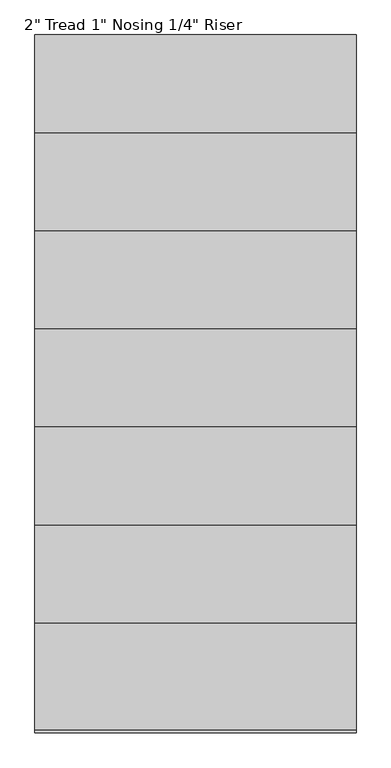
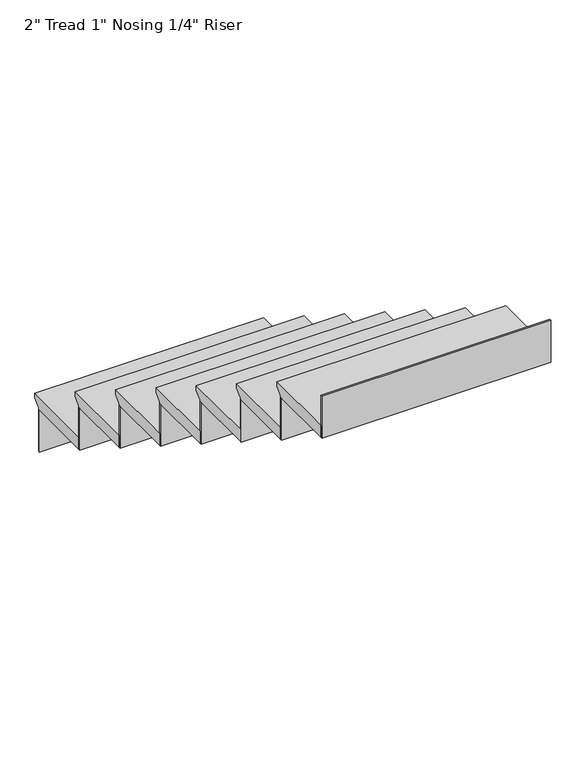
"""IFC4 building model written with IfcOpenShell, lengths in millimetres: stair flight geometry."""

from ifc_helpers import new_model, si_unit, frame, origin, place, context, project, spatial, polyline, outline, extrude, source, transform, mapped, element, save


def stair_flight_4fb3dba1(model_context):
    return source(origin(), model_context, "Body", "SweptSolid", [
        extrude(outline(polyline([(494.0027016, 8966.2), (798.8027016, 8966.2), (798.8027016, 8947.15), (773.4027016, 8921.75), (773.4027016, 8915.4), (494.0027016, 8915.4), (494.0027016, 8966.2)])), frame((8683.6260838, 0.0, 0.0), z_axis=(1.0, 0.0, 0.0), x_axis=(0.0, 1.0, 0.0)), (0.0, 0.0, 1.0), 914.4),
        extrude(outline(polyline([(8683.6260838, 767.0527016), (8683.6260838, 773.4027016), (9598.0260838, 773.4027016), (9598.0260838, 767.0527016), (8683.6260838, 767.0527016)])), frame((0.0, 0.0, 8737.6), z_axis=(0.0, 0.0, 1.0), x_axis=(1.0, 0.0, 0.0)), (0.0, 0.0, 1.0), 177.8),
        extrude(outline(polyline([(8683.6260838, 487.6527016), (8683.6260838, 494.0027016), (9598.0260838, 494.0027016), (9598.0260838, 487.6527016), (8683.6260838, 487.6527016)])), frame((0.0, 0.0, 8915.4), z_axis=(0.0, 0.0, 1.0), x_axis=(1.0, 0.0, 0.0)), (0.0, 0.0, 1.0), 177.8),
        extrude(outline(polyline([(214.6027016, 9144.0), (519.4027016, 9144.0), (519.4027016, 9124.95), (494.0027016, 9099.55), (494.0027016, 9093.2), (214.6027016, 9093.2), (214.6027016, 9144.0)])), frame((8683.6260838, 0.0, 0.0), z_axis=(1.0, 0.0, 0.0), x_axis=(0.0, 1.0, 0.0)), (0.0, 0.0, 1.0), 914.4),
        extrude(outline(polyline([(8683.6260838, 208.2527016), (8683.6260838, 214.6027016), (9598.0260838, 214.6027016), (9598.0260838, 208.2527016), (8683.6260838, 208.2527016)])), frame((0.0, 0.0, 9093.2), z_axis=(0.0, 0.0, 1.0), x_axis=(1.0, 0.0, 0.0)), (0.0, 0.0, 1.0), 177.8),
        extrude(outline(polyline([(-64.7972984, 9321.8), (240.0027016, 9321.8), (240.0027016, 9302.75), (214.6027016, 9277.35), (214.6027016, 9271.0), (-64.7972984, 9271.0), (-64.7972984, 9321.8)])), frame((8683.6260838, 0.0, 0.0), z_axis=(1.0, 0.0, 0.0), x_axis=(0.0, 1.0, 0.0)), (0.0, 0.0, 1.0), 914.4),
        extrude(outline(polyline([(8683.6260838, -71.1472984), (8683.6260838, -64.7972984), (9598.0260838, -64.7972984), (9598.0260838, -71.1472984), (8683.6260838, -71.1472984)])), frame((0.0, 0.0, 9271.0), z_axis=(0.0, 0.0, 1.0), x_axis=(1.0, 0.0, 0.0)), (0.0, 0.0, 1.0), 177.8),
        extrude(outline(polyline([(-344.1972984, 9499.6), (-39.3972984, 9499.6), (-39.3972984, 9480.55), (-64.7972984, 9455.15), (-64.7972984, 9448.8), (-344.1972984, 9448.8), (-344.1972984, 9499.6)])), frame((8683.6260838, 0.0, 0.0), z_axis=(1.0, 0.0, 0.0), x_axis=(0.0, 1.0, 0.0)), (0.0, 0.0, 1.0), 914.4),
        extrude(outline(polyline([(8683.6260838, -350.5472984), (8683.6260838, -344.1972984), (9598.0260838, -344.1972984), (9598.0260838, -350.5472984), (8683.6260838, -350.5472984)])), frame((0.0, 0.0, 9448.8), z_axis=(0.0, 0.0, 1.0), x_axis=(1.0, 0.0, 0.0)), (0.0, 0.0, 1.0), 177.8),
        extrude(outline(polyline([(-623.5972984, 9677.4), (-318.7972984, 9677.4), (-318.7972984, 9658.35), (-344.1972984, 9632.95), (-344.1972984, 9626.6), (-623.5972984, 9626.6), (-623.5972984, 9677.4)])), frame((8683.6260838, 0.0, 0.0), z_axis=(1.0, 0.0, 0.0), x_axis=(0.0, 1.0, 0.0)), (0.0, 0.0, 1.0), 914.4),
        extrude(outline(polyline([(8683.6260838, -629.9472984), (8683.6260838, -623.5972984), (9598.0260838, -623.5972984), (9598.0260838, -629.9472984), (8683.6260838, -629.9472984)])), frame((0.0, 0.0, 9626.6), z_axis=(0.0, 0.0, 1.0), x_axis=(1.0, 0.0, 0.0)), (0.0, 0.0, 1.0), 177.8),
        extrude(outline(polyline([(-902.9972984, 9855.2), (-598.1972984, 9855.2), (-598.1972984, 9836.15), (-623.5972984, 9810.75), (-623.5972984, 9804.4), (-902.9972984, 9804.4), (-902.9972984, 9855.2)])), frame((8683.6260838, 0.0, 0.0), z_axis=(1.0, 0.0, 0.0), x_axis=(0.0, 1.0, 0.0)), (0.0, 0.0, 1.0), 914.4),
        extrude(outline(polyline([(8683.6260838, -909.3472984), (8683.6260838, -902.9972984), (9598.0260838, -902.9972984), (9598.0260838, -909.3472984), (8683.6260838, -909.3472984)])), frame((0.0, 0.0, 9804.4), z_axis=(0.0, 0.0, 1.0), x_axis=(1.0, 0.0, 0.0)), (0.0, 0.0, 1.0), 177.8),
        extrude(outline(polyline([(8683.6260838, -1188.7472984), (8683.6260838, -1182.3972984), (9598.0260838, -1182.3972984), (9598.0260838, -1188.7472984), (8683.6260838, -1188.7472984)])), frame((0.0, 0.0, 9982.2), z_axis=(0.0, 0.0, 1.0), x_axis=(1.0, 0.0, 0.0)), (0.0, 0.0, 1.0), 177.8),
        extrude(outline(polyline([(-1182.3972984, 10033.0), (-877.5972984, 10033.0), (-877.5972984, 10013.95), (-902.9972984, 9988.55), (-902.9972984, 9982.2), (-1182.3972984, 9982.2), (-1182.3972984, 10033.0)])), frame((8683.6260838, 0.0, 0.0), z_axis=(1.0, 0.0, 0.0), x_axis=(0.0, 1.0, 0.0)), (0.0, 0.0, 1.0), 914.4),
    ])


if __name__ == "__main__":
    model = new_model("IFC4")
    model_context = context("Model", 3, world=origin())
    ifc_project = project(units=[si_unit("LENGTHUNIT", "METRE", prefix="MILLI")], contexts=[model_context])
    site = spatial("IfcSite", under=ifc_project)
    building = spatial("IfcBuilding", under=site)
    placement = place(None, origin())
    stair_flight_shape = stair_flight_4fb3dba1(model_context)
    element("IfcStairFlight", 1, ObjectType="2\" Tread 1\" Nosing 1/4\" Riser", at=placement, inside=building, context=model_context, shape_type="MappedRepresentation", body=[
        mapped(stair_flight_shape, transform((0.0, 0.0, 0.0), x_axis=(1.0, 0.0, 0.0), y_axis=(0.0, 1.0, 0.0), z_axis=(0.0, 0.0, 1.0))),
    ])
    save(model, "model.ifc")
